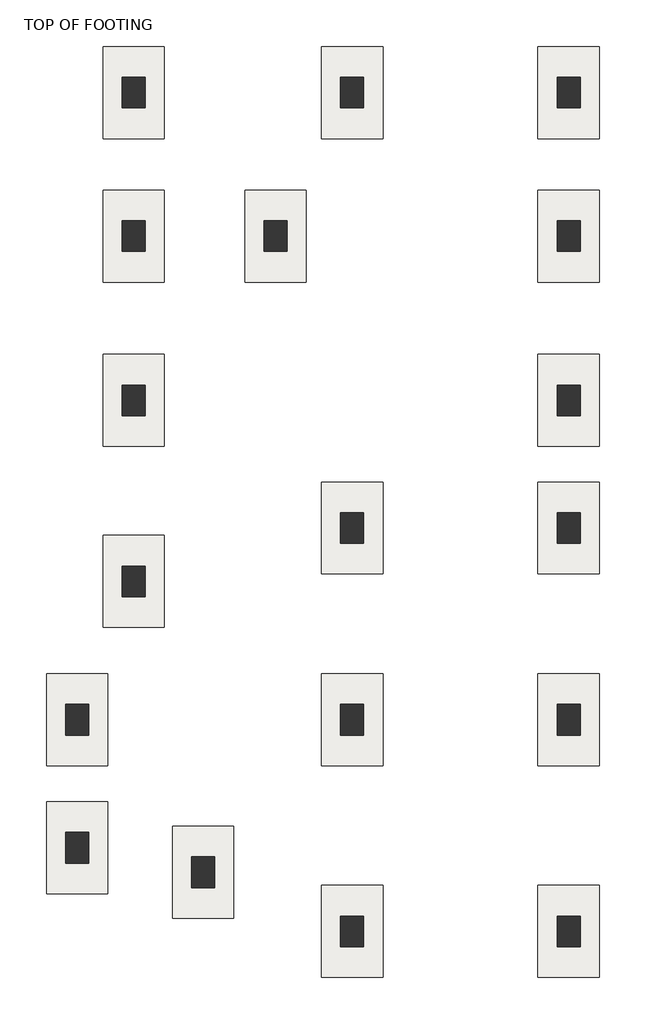
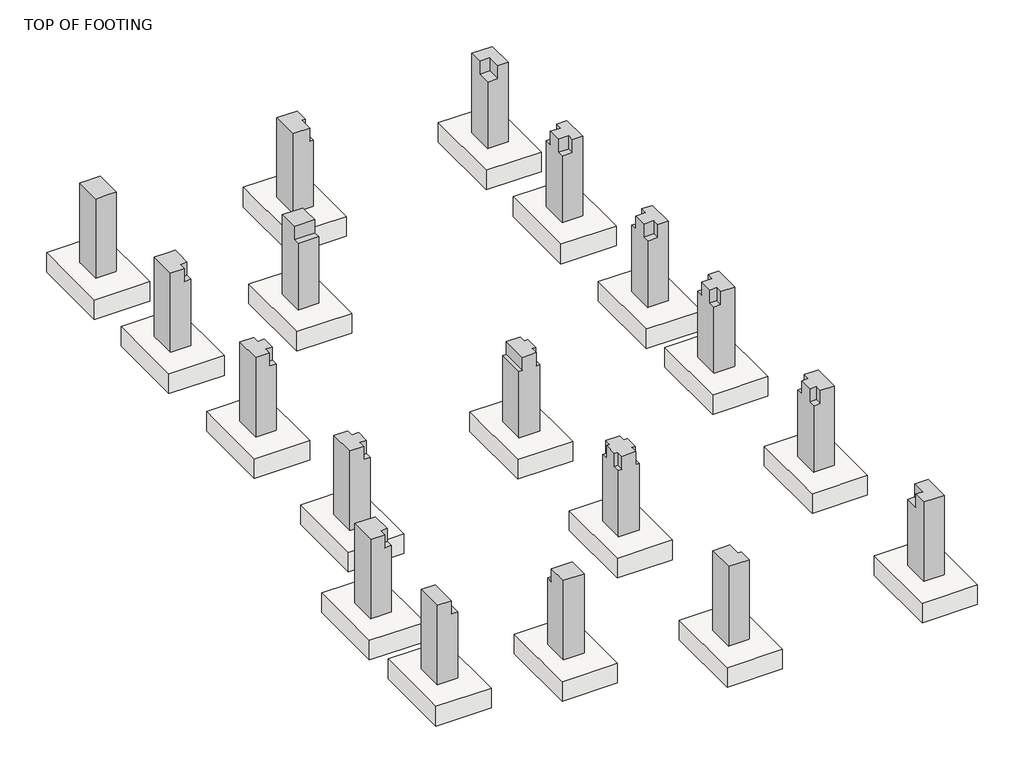
# One storey: 18 columns, 18 slabs.
"""IFC4 building model written with IfcOpenShell, lengths in millimetres."""

from ifc_helpers import new_model, si_unit, frame, origin, place, context, project, spatial, polyline, outline, extrude, faceted_brep, transform, mapped, element, save
from components import m_footing_rectangular_1800_x_1200_x_450mm_16ba7ea5

model = new_model("IFC4")

# Units and contexts
model_context = context("Model", 3, world=origin())
ifc_project = project(units=[si_unit("LENGTHUNIT", "METRE", prefix="MILLI")], contexts=[model_context])

# Site, building, storey
site = spatial("IfcSite", under=ifc_project)
building = spatial("IfcBuilding", under=site)
storey = spatial("IfcBuildingStorey", under=building, Name="TOP OF FOOTING", Elevation=-1828.8)

# Columns
placement = place(None, origin())
element("IfcColumn", 1, ObjectType="M_Concrete-Rectangular-Column : 450 x 600mm", at=placement, inside=storey, context=model_context, shape_type="SweptSolid", body=[
    extrude(outline(polyline([(-1828.8, -7482.9642664), (-1828.8, -7032.9642664), (-300.0, -7032.9642664), (-300.0, -7182.9642664), (0.0, -7182.9642664), (0.0, -7482.9642664), (-1828.8, -7482.9642664)])), frame((0.0, -4929.2575036, 0.0), z_axis=(0.0, 1.0, 0.0), x_axis=(0.0, 0.0, 1.0)), (0.0, 0.0, 1.0), 600.0),
])
element("IfcColumn", 2, ObjectType="M_Concrete-Rectangular-Column : 450 x 600mm", at=placement, inside=storey, context=model_context, shape_type="Brep", body=[
    faceted_brep([(-5925.9642664, 10450.0657956, -1828.8), (-5925.9642664, 9850.0657956, -1828.8), (-6375.9642664, 9850.0657956, -1828.8), (-6375.9642664, 10450.0657956, -1828.8), (-5925.9642664, 10450.0657956, 0.0), (-5925.9642664, 10150.0657956, 0.0), (-5925.9642664, 9850.0657956, 0.0), (-5925.9642664, 9850.0657956, -300.0), (-6075.9642664, 9850.0657956, 0.0), (-6375.9642664, 9850.0657956, 0.0), (-6375.9642664, 10450.0657956, 0.0)], [[[0, 1, 2, 3]], [[1, 0, 4, 5, 6, 7]], [[2, 1, 7, 6, 8, 9]], [[3, 2, 9, 10]], [[0, 3, 10, 4]], [[10, 9, 8, 6, 5, 4]]]),
])
element("IfcColumn", 3, ObjectType="M_Concrete-Rectangular-Column : 450 x 600mm", at=placement, inside=storey, context=model_context, shape_type="Brep", body=[
    faceted_brep([(-5925.9642664, 7641.506653, -1828.8), (-5925.9642664, 7041.506653, -1828.8), (-6375.9642664, 7041.506653, -1828.8), (-6375.9642664, 7641.506653, -1828.8), (-5925.9642664, 7641.506653, -300.0), (-5925.9642664, 7641.506653, 0.0), (-5925.9642664, 7491.506653, 0.0), (-5925.9642664, 7191.506653, 0.0), (-5925.9642664, 7191.506653, -300.0), (-5925.9642664, 7041.506653, -300.0), (-6075.9642664, 7041.506653, -300.0), (-6075.9642664, 7041.506653, 0.0), (-6375.9642664, 7041.506653, 0.0), (-6375.9642664, 7641.506653, 0.0), (-6075.9642664, 7641.506653, 0.0), (-6075.9642664, 7191.506653, 0.0), (-6075.9642664, 7191.506653, -300.0)], [[[0, 1, 2, 3]], [[1, 0, 4, 5, 6, 7, 8, 9]], [[2, 1, 9, 10, 11, 12]], [[3, 2, 12, 13]], [[0, 3, 13, 14, 5, 4]], [[13, 12, 11, 15, 7, 6, 5, 14]], [[16, 10, 9, 8]], [[15, 16, 8, 7]], [[16, 15, 11, 10]]]),
])
element("IfcColumn", 4, ObjectType="M_Concrete-Rectangular-Column : 450 x 600mm", at=placement, inside=storey, context=model_context, shape_type="Brep", body=[
    faceted_brep([(-5925.9642664, 4424.5351605, -1828.8), (-5925.9642664, 3824.5351605, -1828.8), (-6375.9642664, 3824.5351605, -1828.8), (-6375.9642664, 4424.5351605, -1828.8), (-5925.9642664, 4424.5351605, -300.0), (-5925.9642664, 4274.5351605, -300.0), (-5925.9642664, 4274.5351605, 0.0), (-5925.9642664, 3974.5351605, 0.0), (-5925.9642664, 3974.5351605, -300.0), (-5925.9642664, 3824.5351605, -300.0), (-6075.9642664, 3824.5351605, -300.0), (-6075.9642664, 3824.5351605, 0.0), (-6375.9642664, 3824.5351605, 0.0), (-6375.9642664, 4424.5351605, 0.0), (-6075.9642664, 4424.5351605, 0.0), (-6075.9642664, 4424.5351605, -300.0), (-6075.9642664, 3974.5351605, 0.0), (-6075.9642664, 4274.5351605, 0.0), (-6075.9642664, 4274.5351605, -300.0), (-6075.9642664, 3974.5351605, -300.0)], [[[0, 1, 2, 3]], [[1, 0, 4, 5, 6, 7, 8, 9]], [[2, 1, 9, 10, 11, 12]], [[3, 2, 12, 13]], [[0, 3, 13, 14, 15, 4]], [[13, 12, 11, 16, 7, 6, 17, 14]], [[15, 18, 5, 4]], [[18, 17, 6, 5]], [[17, 18, 15, 14]], [[19, 10, 9, 8]], [[16, 19, 8, 7]], [[19, 16, 11, 10]]]),
])
element("IfcColumn", 5, ObjectType="M_Concrete-Rectangular-Column : 450 x 600mm", at=placement, inside=storey, context=model_context, shape_type="Brep", body=[
    faceted_brep([(-5925.9642664, 881.5941646, -1828.8), (-5925.9642664, 281.5941646, -1828.8), (-6375.9642664, 281.5941646, -1828.8), (-6375.9642664, 881.5941646, -1828.8), (-5925.9642664, 881.5941646, -300.0), (-5925.9642664, 731.5941646, -300.0), (-5925.9642664, 731.5941646, 0.0), (-5925.9642664, 431.5941646, 0.0), (-5925.9642664, 431.5941646, -300.0), (-5925.9642664, 281.5941646, -300.0), (-6075.9642664, 281.5941646, -300.0), (-6075.9642664, 281.5941646, 0.0), (-6375.9642664, 281.5941646, 0.0), (-6375.9642664, 881.5941646, 0.0), (-6075.9642664, 881.5941646, 0.0), (-6075.9642664, 881.5941646, -300.0), (-6075.9642664, 431.5941646, 0.0), (-6075.9642664, 731.5941646, 0.0), (-6075.9642664, 731.5941646, -300.0), (-6075.9642664, 431.5941646, -300.0)], [[[0, 1, 2, 3]], [[1, 0, 4, 5, 6, 7, 8, 9]], [[2, 1, 9, 10, 11, 12]], [[3, 2, 12, 13]], [[0, 3, 13, 14, 15, 4]], [[13, 12, 11, 16, 7, 6, 17, 14]], [[15, 18, 5, 4]], [[18, 17, 6, 5]], [[17, 18, 15, 14]], [[19, 10, 9, 8]], [[19, 16, 11, 10]], [[16, 19, 8, 7]]]),
])
element("IfcColumn", 6, ObjectType="M_Concrete-Rectangular-Column : 450 x 600mm", at=placement, inside=storey, context=model_context, shape_type="Brep", body=[
    faceted_brep([(-3146.635935, 7641.506653, -1828.8), (-3146.635935, 7041.506653, -1828.8), (-3596.635935, 7041.506653, -1828.8), (-3596.635935, 7641.506653, -1828.8), (-3146.635935, 7641.506653, -300.0), (-3146.635935, 7641.506653, 0.0), (-3146.635935, 7491.506653, 0.0), (-3146.635935, 7191.506653, 0.0), (-3146.635935, 7191.506653, -300.0), (-3146.635935, 7041.506653, -300.0), (-3596.635935, 7041.506653, -300.0), (-3596.635935, 7191.506653, -300.0), (-3596.635935, 7191.506653, 0.0), (-3596.635935, 7491.506653, 0.0), (-3596.635935, 7641.506653, 0.0), (-3596.635935, 7641.506653, -300.0)], [[[0, 1, 2, 3]], [[1, 0, 4, 5, 6, 7, 8, 9]], [[2, 1, 9, 10]], [[3, 2, 10, 11, 12, 13, 14, 15]], [[0, 3, 15, 14, 5, 4]], [[5, 14, 13, 12, 7, 6]], [[8, 11, 10, 9]], [[11, 8, 7, 12]]]),
])
element("IfcColumn", 7, ObjectType="M_Concrete-Rectangular-Column : 450 x 600mm", at=placement, inside=storey, context=model_context, shape_type="Brep", body=[
    faceted_brep([(-1646.635935, 10450.0657956, -1828.8), (-1646.635935, 9850.0657956, -1828.8), (-2096.635935, 9850.0657956, -1828.8), (-2096.635935, 10450.0657956, -1828.8), (-1646.635935, 10450.0657956, 0.0), (-1646.635935, 10150.0657956, 0.0), (-1646.635935, 10150.0657956, -300.0), (-1646.635935, 9850.0657956, -300.0), (-1721.635935, 9850.0657956, -300.0), (-1721.635935, 9850.0657956, 0.0), (-2021.635935, 9850.0657956, 0.0), (-2096.635935, 9850.0657956, 0.0), (-2096.635935, 9850.0657956, -300.0), (-2096.635935, 10150.0657956, 0.0), (-2096.635935, 10450.0657956, 0.0), (-1721.635935, 10150.0657956, 0.0), (-1721.635935, 10150.0657956, -300.0)], [[[0, 1, 2, 3]], [[1, 0, 4, 5, 6, 7]], [[2, 1, 7, 8, 9, 10, 11, 12]], [[3, 2, 12, 11, 13, 14]], [[0, 3, 14, 4]], [[4, 14, 13, 11, 10, 9, 15, 5]], [[16, 8, 7, 6]], [[15, 16, 6, 5]], [[16, 15, 9, 8]]]),
])
element("IfcColumn", 8, ObjectType="M_Concrete-Rectangular-Column : 450 x 600mm", at=placement, inside=storey, context=model_context, shape_type="Brep", body=[
    faceted_brep([(-1646.635935, 1928.1057379, -1828.8), (-1646.635935, 1328.1057379, -1828.8), (-2096.635935, 1328.1057379, -1828.8), (-2096.635935, 1928.1057379, -1828.8), (-1646.635935, 1928.1057379, -300.0), (-1646.635935, 1778.1057379, -300.0), (-1646.635935, 1778.1057379, 0.0), (-1646.635935, 1478.1057379, 0.0), (-1646.635935, 1478.1057379, -300.0), (-1646.635935, 1328.1057379, -300.0), (-1721.635935, 1328.1057379, -300.0), (-1721.635935, 1328.1057379, 0.0), (-2021.635935, 1328.1057379, 0.0), (-2021.635935, 1328.1057379, -300.0), (-2096.635935, 1328.1057379, -300.0), (-2096.635935, 1928.1057379, -300.0), (-2021.635935, 1928.1057379, -300.0), (-2021.635935, 1928.1057379, 0.0), (-1721.635935, 1928.1057379, 0.0), (-1721.635935, 1928.1057379, -300.0), (-1721.635935, 1778.1057379, 0.0), (-1721.635935, 1478.1057379, 0.0), (-1721.635935, 1778.1057379, -300.0), (-1721.635935, 1478.1057379, -300.0)], [[[0, 1, 2, 3]], [[1, 0, 4, 5, 6, 7, 8, 9]], [[2, 1, 9, 10, 11, 12, 13, 14]], [[3, 2, 14, 15]], [[0, 3, 15, 16, 17, 18, 19, 4]], [[6, 20, 18, 17, 12, 11, 21, 7]], [[19, 22, 5, 4]], [[22, 20, 6, 5]], [[20, 22, 19, 18]], [[23, 10, 9, 8]], [[21, 23, 8, 7]], [[23, 21, 11, 10]], [[13, 16, 15, 14]], [[16, 13, 12, 17]]]),
])
element("IfcColumn", 9, ObjectType="M_Concrete-Rectangular-Column : 450 x 600mm", at=placement, inside=storey, context=model_context, shape_type="Brep", body=[
    faceted_brep([(-1646.635935, -1823.3693625, -1828.8), (-1646.635935, -2423.3693625, -1828.8), (-2096.635935, -2423.3693625, -1828.8), (-2096.635935, -1823.3693625, -1828.8), (-1646.635935, -1823.3693625, -300.0), (-1646.635935, -1973.3693625, -300.0), (-1646.635935, -1973.3693625, 0.0), (-1646.635935, -2273.3693625, 0.0), (-1646.635935, -2273.3693625, -300.0), (-1646.635935, -2423.3693625, -300.0), (-1721.635935, -2423.3693625, -300.0), (-1721.635935, -2423.3693625, 0.0), (-2021.635935, -2423.3693625, 0.0), (-2021.635935, -2423.3693625, -300.0), (-2096.635935, -2423.3693625, -300.0), (-2096.635935, -2273.3693625, -300.0), (-2096.635935, -2273.3693625, 0.0), (-2096.635935, -1973.3693625, 0.0), (-2096.635935, -1973.3693625, -300.0), (-2096.635935, -1823.3693625, -300.0), (-2021.635935, -1823.3693625, -300.0), (-2021.635935, -1823.3693625, 0.0), (-1721.635935, -1823.3693625, 0.0), (-1721.635935, -1823.3693625, -300.0), (-1721.635935, -1973.3693625, 0.0), (-2021.635935, -1973.3693625, 0.0), (-2021.635935, -2273.3693625, 0.0), (-1721.635935, -2273.3693625, 0.0), (-1721.635935, -1973.3693625, -300.0), (-1721.635935, -2273.3693625, -300.0), (-2021.635935, -1973.3693625, -300.0), (-2021.635935, -2273.3693625, -300.0)], [[[0, 1, 2, 3]], [[1, 0, 4, 5, 6, 7, 8, 9]], [[2, 1, 9, 10, 11, 12, 13, 14]], [[3, 2, 14, 15, 16, 17, 18, 19]], [[0, 3, 19, 20, 21, 22, 23, 4]], [[6, 24, 22, 21, 25, 17, 16, 26, 12, 11, 27, 7]], [[23, 28, 5, 4]], [[28, 24, 6, 5]], [[24, 28, 23, 22]], [[29, 10, 9, 8]], [[27, 29, 8, 7]], [[29, 27, 11, 10]], [[18, 30, 20, 19]], [[30, 25, 21, 20]], [[25, 30, 18, 17]], [[13, 31, 15, 14]], [[31, 26, 16, 15]], [[26, 31, 13, 12]]]),
])
element("IfcColumn", 10, ObjectType="M_Concrete-Rectangular-Column : 450 x 600mm", at=placement, inside=storey, context=model_context, shape_type="Brep", body=[
    faceted_brep([(-1646.635935, -5967.3380763, -1828.8), (-1646.635935, -6567.3380763, -1828.8), (-2096.635935, -6567.3380763, -1828.8), (-2096.635935, -5967.3380763, -1828.8), (-1646.635935, -5967.3380763, -300.0), (-1646.635935, -6267.3380763, -300.0), (-1646.635935, -6267.3380763, 0.0), (-1646.635935, -6567.3380763, 0.0), (-2096.635935, -6567.3380763, 0.0), (-2096.635935, -5967.3380763, 0.0), (-1721.635935, -5967.3380763, 0.0), (-1721.635935, -5967.3380763, -300.0), (-1721.635935, -6267.3380763, 0.0), (-1721.635935, -6267.3380763, -300.0)], [[[0, 1, 2, 3]], [[1, 0, 4, 5, 6, 7]], [[2, 1, 7, 8]], [[3, 2, 8, 9]], [[0, 3, 9, 10, 11, 4]], [[8, 7, 6, 12, 10, 9]], [[11, 13, 5, 4]], [[13, 12, 6, 5]], [[12, 13, 11, 10]]]),
])
element("IfcColumn", 11, ObjectType="M_Concrete-Rectangular-Column : 450 x 600mm", at=placement, inside=storey, context=model_context, shape_type="Brep", body=[
    faceted_brep([(2593.5134108, 10450.0657956, -1828.8), (2593.5134108, 9850.0657956, -1828.8), (2143.5134108, 9850.0657956, -1828.8), (2143.5134108, 10450.0657956, -1828.8), (2593.5134108, 10450.0657956, 0.0), (2593.5134108, 9850.0657956, 0.0), (2368.5134108, 9850.0657956, 0.0), (2368.5134108, 9850.0657956, -300.0), (2143.5134108, 9850.0657956, -300.0), (2143.5134108, 10150.0657956, -300.0), (2143.5134108, 10150.0657956, 0.0), (2143.5134108, 10450.0657956, 0.0), (2368.5134108, 10150.0657956, 0.0), (2368.5134108, 10150.0657956, -300.0)], [[[0, 1, 2, 3]], [[1, 0, 4, 5]], [[2, 1, 5, 6, 7, 8]], [[3, 2, 8, 9, 10, 11]], [[0, 3, 11, 4]], [[5, 4, 11, 10, 12, 6]], [[7, 13, 9, 8]], [[13, 12, 10, 9]], [[12, 13, 7, 6]]]),
])
element("IfcColumn", 12, ObjectType="M_Concrete-Rectangular-Column : 450 x 600mm", at=placement, inside=storey, context=model_context, shape_type="Brep", body=[
    faceted_brep([(2593.5134108, 7641.506653, -1828.8), (2593.5134108, 7041.506653, -1828.8), (2143.5134108, 7041.506653, -1828.8), (2143.5134108, 7641.506653, -1828.8), (2593.5134108, 7641.506653, 0.0), (2593.5134108, 7041.506653, 0.0), (2368.5134108, 7041.506653, 0.0), (2368.5134108, 7041.506653, -300.0), (2143.5134108, 7041.506653, -300.0), (2143.5134108, 7191.506653, -300.0), (2143.5134108, 7191.506653, 0.0), (2143.5134108, 7491.506653, 0.0), (2143.5134108, 7491.506653, -300.0), (2143.5134108, 7641.506653, -300.0), (2368.5134108, 7641.506653, -300.0), (2368.5134108, 7641.506653, 0.0), (2368.5134108, 7491.506653, 0.0), (2368.5134108, 7191.506653, 0.0), (2368.5134108, 7491.506653, -300.0), (2368.5134108, 7191.506653, -300.0)], [[[0, 1, 2, 3]], [[1, 0, 4, 5]], [[2, 1, 5, 6, 7, 8]], [[3, 2, 8, 9, 10, 11, 12, 13]], [[0, 3, 13, 14, 15, 4]], [[5, 4, 15, 16, 11, 10, 17, 6]], [[12, 18, 14, 13]], [[18, 16, 15, 14]], [[16, 18, 12, 11]], [[7, 19, 9, 8]], [[19, 17, 10, 9]], [[17, 19, 7, 6]]]),
])
element("IfcColumn", 13, ObjectType="M_Concrete-Rectangular-Column : 450 x 600mm", at=placement, inside=storey, context=model_context, shape_type="Brep", body=[
    faceted_brep([(2593.5134108, 4424.5351605, -1828.8), (2593.5134108, 3824.5351605, -1828.8), (2143.5134108, 3824.5351605, -1828.8), (2143.5134108, 4424.5351605, -1828.8), (2593.5134108, 4424.5351605, 0.0), (2593.5134108, 3824.5351605, 0.0), (2368.5134108, 3824.5351605, 0.0), (2368.5134108, 3824.5351605, -300.0), (2143.5134108, 3824.5351605, -300.0), (2143.5134108, 3974.5351605, -300.0), (2143.5134108, 3974.5351605, 0.0), (2143.5134108, 4274.5351605, 0.0), (2143.5134108, 4274.5351605, -300.0), (2143.5134108, 4424.5351605, -300.0), (2368.5134108, 4424.5351605, -300.0), (2368.5134108, 4424.5351605, 0.0), (2368.5134108, 4274.5351605, 0.0), (2368.5134108, 3974.5351605, 0.0), (2368.5134108, 4274.5351605, -300.0), (2368.5134108, 3974.5351605, -300.0)], [[[0, 1, 2, 3]], [[1, 0, 4, 5]], [[2, 1, 5, 6, 7, 8]], [[3, 2, 8, 9, 10, 11, 12, 13]], [[0, 3, 13, 14, 15, 4]], [[5, 4, 15, 16, 11, 10, 17, 6]], [[12, 18, 14, 13]], [[18, 16, 15, 14]], [[16, 18, 12, 11]], [[7, 19, 9, 8]], [[17, 19, 7, 6]], [[19, 17, 10, 9]]]),
])
element("IfcColumn", 14, ObjectType="M_Concrete-Rectangular-Column : 450 x 600mm", at=placement, inside=storey, context=model_context, shape_type="Brep", body=[
    faceted_brep([(2593.5134108, 1928.1057379, -1828.8), (2593.5134108, 1328.1057379, -1828.8), (2143.5134108, 1328.1057379, -1828.8), (2143.5134108, 1928.1057379, -1828.8), (2593.5134108, 1928.1057379, 0.0), (2593.5134108, 1328.1057379, 0.0), (2293.5134108, 1328.1057379, 0.0), (2293.5134108, 1328.1057379, -300.0), (2143.5134108, 1328.1057379, -300.0), (2143.5134108, 1478.1057379, -300.0), (2143.5134108, 1478.1057379, 0.0), (2143.5134108, 1778.1057379, 0.0), (2143.5134108, 1778.1057379, -300.0), (2143.5134108, 1928.1057379, -300.0), (2368.5134108, 1928.1057379, -300.0), (2368.5134108, 1928.1057379, 0.0), (2368.5134108, 1778.1057379, 0.0), (2293.5134108, 1478.1057379, 0.0), (2368.5134108, 1778.1057379, -300.0), (2293.5134108, 1478.1057379, -300.0)], [[[0, 1, 2, 3]], [[1, 0, 4, 5]], [[2, 1, 5, 6, 7, 8]], [[3, 2, 8, 9, 10, 11, 12, 13]], [[0, 3, 13, 14, 15, 4]], [[5, 4, 15, 16, 11, 10, 17, 6]], [[12, 18, 14, 13]], [[18, 16, 15, 14]], [[16, 18, 12, 11]], [[7, 19, 9, 8]], [[19, 17, 10, 9]], [[17, 19, 7, 6]]]),
])
element("IfcColumn", 15, ObjectType="M_Concrete-Rectangular-Column : 450 x 600mm", at=placement, inside=storey, context=model_context, shape_type="Brep", body=[
    faceted_brep([(2593.5134108, -1823.3693625, -1828.8), (2593.5134108, -2423.3693625, -1828.8), (2143.5134108, -2423.3693625, -1828.8), (2143.5134108, -1823.3693625, -1828.8), (2593.5134108, -1823.3693625, 0.0), (2593.5134108, -2423.3693625, 0.0), (2293.5134108, -2423.3693625, 0.0), (2293.5134108, -2423.3693625, -300.0), (2143.5134108, -2423.3693625, -300.0), (2143.5134108, -2273.3693625, -300.0), (2143.5134108, -2273.3693625, 0.0), (2143.5134108, -1973.3693625, 0.0), (2143.5134108, -1973.3693625, -300.0), (2143.5134108, -1823.3693625, -300.0), (2293.5134108, -1823.3693625, -300.0), (2293.5134108, -1823.3693625, 0.0), (2293.5134108, -1973.3693625, 0.0), (2293.5134108, -2273.3693625, 0.0), (2293.5134108, -1973.3693625, -300.0), (2293.5134108, -2273.3693625, -300.0)], [[[0, 1, 2, 3]], [[1, 0, 4, 5]], [[2, 1, 5, 6, 7, 8]], [[3, 2, 8, 9, 10, 11, 12, 13]], [[0, 3, 13, 14, 15, 4]], [[5, 4, 15, 16, 11, 10, 17, 6]], [[12, 18, 14, 13]], [[18, 16, 15, 14]], [[16, 18, 12, 11]], [[7, 19, 9, 8]], [[19, 17, 10, 9]], [[17, 19, 7, 6]]]),
])
element("IfcColumn", 16, ObjectType="M_Concrete-Rectangular-Column : 450 x 600mm", at=placement, inside=storey, context=model_context, shape_type="Brep", body=[
    faceted_brep([(2593.5134108, -5967.3380763, -1828.8), (2593.5134108, -6567.3380763, -1828.8), (2143.5134108, -6567.3380763, -1828.8), (2143.5134108, -5967.3380763, -1828.8), (2593.5134108, -5967.3380763, 0.0), (2593.5134108, -6567.3380763, 0.0), (2143.5134108, -6567.3380763, 0.0), (2143.5134108, -6267.3380763, 0.0), (2143.5134108, -6267.3380763, -300.0), (2143.5134108, -5967.3380763, -300.0), (2293.5134108, -5967.3380763, -300.0), (2293.5134108, -5967.3380763, 0.0), (2293.5134108, -6267.3380763, 0.0), (2293.5134108, -6267.3380763, -300.0)], [[[0, 1, 2, 3]], [[1, 0, 4, 5]], [[2, 1, 5, 6]], [[3, 2, 6, 7, 8, 9]], [[0, 3, 9, 10, 11, 4]], [[5, 4, 11, 12, 7, 6]], [[8, 13, 10, 9]], [[13, 12, 11, 10]], [[12, 13, 8, 7]]]),
])
element("IfcColumn", 17, ObjectType="M_Concrete-Rectangular-Column : 450 x 600mm", at=placement, inside=storey, context=model_context, shape_type="SweptSolid", body=[
    extrude(outline(polyline([(-4809.2575036, -1828.8), (-5409.2575036, -1828.8), (-5409.2575036, 0.0), (-4959.2575036, 0.0), (-4959.2575036, -300.0), (-4809.2575036, -300.0), (-4809.2575036, -1828.8)])), frame((-5016.635935, 0.0, 0.0), z_axis=(1.0, 0.0, 0.0), x_axis=(0.0, 1.0, 0.0)), (0.0, 0.0, 1.0), 450.0),
])
element("IfcColumn", 18, ObjectType="M_Concrete-Rectangular-Column : 450 x 600mm", at=placement, inside=storey, context=model_context, shape_type="Brep", body=[
    faceted_brep([(-7032.9642664, -1823.3693625, -1828.8), (-7032.9642664, -2423.3693625, -1828.8), (-7482.9642664, -2423.3693625, -1828.8), (-7482.9642664, -1823.3693625, -1828.8), (-7032.9642664, -1823.3693625, 0.0), (-7032.9642664, -2273.3693625, 0.0), (-7032.9642664, -2273.3693625, -300.0), (-7032.9642664, -2423.3693625, -300.0), (-7182.9642664, -2423.3693625, -300.0), (-7182.9642664, -2423.3693625, 0.0), (-7482.9642664, -2423.3693625, 0.0), (-7482.9642664, -1823.3693625, 0.0), (-7182.9642664, -2273.3693625, 0.0), (-7182.9642664, -2273.3693625, -300.0)], [[[0, 1, 2, 3]], [[1, 0, 4, 5, 6, 7]], [[2, 1, 7, 8, 9, 10]], [[3, 2, 10, 11]], [[0, 3, 11, 4]], [[11, 10, 9, 12, 5, 4]], [[13, 8, 7, 6]], [[12, 13, 6, 5]], [[13, 12, 9, 8]]]),
])

# Slabs
m_footing_rectangular_1800_x_1200_x_450mm_shape = m_footing_rectangular_1800_x_1200_x_450mm_16ba7ea5(model_context)
element("IfcSlab", 19, ObjectType="M_Footing-Rectangular : 1800 x 1200 x 450mm", at=placement, inside=storey, context=model_context, shape_type="MappedRepresentation", body=[
    mapped(m_footing_rectangular_1800_x_1200_x_450mm_shape, transform((-7257.9642664, -4629.2575036, -1828.8), x_axis=(1.0, 0.0, 0.0), y_axis=(0.0, 1.0, 0.0), z_axis=(0.0, 0.0, 1.0))),
])
element("IfcSlab", 20, ObjectType="M_Footing-Rectangular : 1800 x 1200 x 450mm", at=placement, inside=storey, context=model_context, shape_type="MappedRepresentation", body=[
    mapped(m_footing_rectangular_1800_x_1200_x_450mm_shape, transform((-4791.635935, -5109.2575036, -1828.8), x_axis=(1.0, 0.0, 0.0), y_axis=(0.0, 1.0, 0.0), z_axis=(0.0, 0.0, 1.0))),
])
element("IfcSlab", 21, ObjectType="M_Footing-Rectangular : 1800 x 1200 x 450mm", at=placement, inside=storey, context=model_context, shape_type="MappedRepresentation", body=[
    mapped(m_footing_rectangular_1800_x_1200_x_450mm_shape, transform((2368.5134108, -6267.3380763, -1828.8), x_axis=(1.0, 0.0, 0.0), y_axis=(0.0, 1.0, 0.0), z_axis=(0.0, 0.0, 1.0))),
])
element("IfcSlab", 22, ObjectType="M_Footing-Rectangular : 1800 x 1200 x 450mm", at=placement, inside=storey, context=model_context, shape_type="MappedRepresentation", body=[
    mapped(m_footing_rectangular_1800_x_1200_x_450mm_shape, transform((-1871.635935, -6267.3380763, -1828.8), x_axis=(1.0, 0.0, 0.0), y_axis=(0.0, 1.0, 0.0), z_axis=(0.0, 0.0, 1.0))),
])
element("IfcSlab", 23, ObjectType="M_Footing-Rectangular : 1800 x 1200 x 450mm", at=placement, inside=storey, context=model_context, shape_type="MappedRepresentation", body=[
    mapped(m_footing_rectangular_1800_x_1200_x_450mm_shape, transform((2368.5134108, -2123.3693625, -1828.8), x_axis=(1.0, 0.0, 0.0), y_axis=(0.0, 1.0, 0.0), z_axis=(0.0, 0.0, 1.0))),
])
element("IfcSlab", 24, ObjectType="M_Footing-Rectangular : 1800 x 1200 x 450mm", at=placement, inside=storey, context=model_context, shape_type="MappedRepresentation", body=[
    mapped(m_footing_rectangular_1800_x_1200_x_450mm_shape, transform((2368.5134108, 4124.5351605, -1828.8), x_axis=(1.0, 0.0, 0.0), y_axis=(0.0, 1.0, 0.0), z_axis=(0.0, 0.0, 1.0))),
])
element("IfcSlab", 25, ObjectType="M_Footing-Rectangular : 1800 x 1200 x 450mm", at=placement, inside=storey, context=model_context, shape_type="MappedRepresentation", body=[
    mapped(m_footing_rectangular_1800_x_1200_x_450mm_shape, transform((2368.5134108, 10150.0657956, -1828.8), x_axis=(1.0, 0.0, 0.0), y_axis=(0.0, 1.0, 0.0), z_axis=(0.0, 0.0, 1.0))),
])
element("IfcSlab", 26, ObjectType="M_Footing-Rectangular : 1800 x 1200 x 450mm", at=placement, inside=storey, context=model_context, shape_type="MappedRepresentation", body=[
    mapped(m_footing_rectangular_1800_x_1200_x_450mm_shape, transform((-6150.9642664, 10150.0657956, -1828.8), x_axis=(1.0, 0.0, 0.0), y_axis=(0.0, 1.0, 0.0), z_axis=(0.0, 0.0, 1.0))),
])
element("IfcSlab", 27, ObjectType="M_Footing-Rectangular : 1800 x 1200 x 450mm", at=placement, inside=storey, context=model_context, shape_type="MappedRepresentation", body=[
    mapped(m_footing_rectangular_1800_x_1200_x_450mm_shape, transform((-1871.635935, 10150.0657956, -1828.8), x_axis=(1.0, 0.0, 0.0), y_axis=(0.0, 1.0, 0.0), z_axis=(0.0, 0.0, 1.0))),
])
element("IfcSlab", 28, ObjectType="M_Footing-Rectangular : 1800 x 1200 x 450mm", at=placement, inside=storey, context=model_context, shape_type="MappedRepresentation", body=[
    mapped(m_footing_rectangular_1800_x_1200_x_450mm_shape, transform((-6150.9642664, 581.5941646, -1828.8), x_axis=(1.0, 0.0, 0.0), y_axis=(0.0, 1.0, 0.0), z_axis=(0.0, 0.0, 1.0))),
])
element("IfcSlab", 29, ObjectType="M_Footing-Rectangular : 1800 x 1200 x 450mm", at=placement, inside=storey, context=model_context, shape_type="MappedRepresentation", body=[
    mapped(m_footing_rectangular_1800_x_1200_x_450mm_shape, transform((-6150.9642664, 4124.5351605, -1828.8), x_axis=(1.0, 0.0, 0.0), y_axis=(0.0, 1.0, 0.0), z_axis=(0.0, 0.0, 1.0))),
])
element("IfcSlab", 30, ObjectType="M_Footing-Rectangular : 1800 x 1200 x 450mm", at=placement, inside=storey, context=model_context, shape_type="MappedRepresentation", body=[
    mapped(m_footing_rectangular_1800_x_1200_x_450mm_shape, transform((-6150.9642664, 7341.506653, -1828.8), x_axis=(1.0, 0.0, 0.0), y_axis=(0.0, 1.0, 0.0), z_axis=(0.0, 0.0, 1.0))),
])
element("IfcSlab", 31, ObjectType="M_Footing-Rectangular : 1800 x 1200 x 450mm", at=placement, inside=storey, context=model_context, shape_type="MappedRepresentation", body=[
    mapped(m_footing_rectangular_1800_x_1200_x_450mm_shape, transform((-3371.635935, 7341.506653, -1828.8), x_axis=(1.0, 0.0, 0.0), y_axis=(0.0, 1.0, 0.0), z_axis=(0.0, 0.0, 1.0))),
])
element("IfcSlab", 32, ObjectType="M_Footing-Rectangular : 1800 x 1200 x 450mm", at=placement, inside=storey, context=model_context, shape_type="MappedRepresentation", body=[
    mapped(m_footing_rectangular_1800_x_1200_x_450mm_shape, transform((2368.5134108, 7341.506653, -1828.8), x_axis=(1.0, 0.0, 0.0), y_axis=(0.0, 1.0, 0.0), z_axis=(0.0, 0.0, 1.0))),
])
element("IfcSlab", 33, ObjectType="M_Footing-Rectangular : 1800 x 1200 x 450mm", at=placement, inside=storey, context=model_context, shape_type="MappedRepresentation", body=[
    mapped(m_footing_rectangular_1800_x_1200_x_450mm_shape, transform((-1871.635935, -2123.3693625, -1828.8), x_axis=(1.0, 0.0, 0.0), y_axis=(0.0, 1.0, 0.0), z_axis=(0.0, 0.0, 1.0))),
])
element("IfcSlab", 34, ObjectType="M_Footing-Rectangular : 1800 x 1200 x 450mm", at=placement, inside=storey, context=model_context, shape_type="MappedRepresentation", body=[
    mapped(m_footing_rectangular_1800_x_1200_x_450mm_shape, transform((2368.5134108, 1628.1057379, -1828.8), x_axis=(1.0, 0.0, 0.0), y_axis=(0.0, 1.0, 0.0), z_axis=(0.0, 0.0, 1.0))),
])
element("IfcSlab", 35, ObjectType="M_Footing-Rectangular : 1800 x 1200 x 450mm", at=placement, inside=storey, context=model_context, shape_type="MappedRepresentation", body=[
    mapped(m_footing_rectangular_1800_x_1200_x_450mm_shape, transform((-1871.635935, 1628.1057379, -1828.8), x_axis=(1.0, 0.0, 0.0), y_axis=(0.0, 1.0, 0.0), z_axis=(0.0, 0.0, 1.0))),
])
element("IfcSlab", 36, ObjectType="M_Footing-Rectangular : 1800 x 1200 x 450mm", at=placement, inside=storey, context=model_context, shape_type="MappedRepresentation", body=[
    mapped(m_footing_rectangular_1800_x_1200_x_450mm_shape, transform((-7257.9642664, -2123.3693625, -1828.8), x_axis=(1.0, 0.0, 0.0), y_axis=(0.0, 1.0, 0.0), z_axis=(0.0, 0.0, 1.0))),
])

save(model, "model.ifc")

# Revit data of these elements
# Grids (mm)
#   "9": line (6345.331, -5109.258) -> (-9404.782, -5109.258)
#   "10": line (6345.331, -6267.338) -> (-9427.998, -6267.338)
#   "1": line (6418.05, 10150.066) -> (-9427.998, 10150.066)
#   "A": line (-7257.964, 12244.334) -> (-7257.964, -11102.212)
#   "B": line (-6150.964, 12244.334) -> (-6150.964, -11102.212)
#   "C": line (-4791.636, 12244.334) -> (-4791.636, -8322.372)
#   "D": line (-3371.636, 12244.334) -> (-3371.636, -8322.372)
#   "2": line (6418.05, 7341.507) -> (-9427.998, 7341.507)
#   "E": line (-1871.636, 12244.334) -> (-1871.636, -8322.372)
#   "F": line (2368.513, 12244.334) -> (2368.513, -8382.306)
#   "8": line (6418.05, -4629.258) -> (-9404.782, -4629.258)
#   "3": line (6418.05, 6151.507) -> (-9427.998, 6151.507)
#   "G": line (3608.513, 12244.334) -> (3608.513, -8322.372)
#   "4": line (6418.05, 4124.535) -> (-9404.782, 4124.535)
#   "5": line (6345.331, 1628.106) -> (-9404.782, 1628.106)
#   "6": line (6345.331, 581.594) -> (-9427.998, 581.594)
#   "7": line (6418.05, -2123.369) -> (-9404.782, -2123.369)
# Type "M_Concrete-Rectangular-Column : 450 x 600mm"
#   b = 450 mm
#   h = 600 mm
#   Structural Material [instance default] = Concrete, Cast-in-Place gray
# Type "M_Footing-Rectangular : 1800 x 1200 x 450mm"
#   Width = 1200 mm
#   Length = 1800 mm
#   Foundation Thickness = 450 mm
#   Structural Material [instance default] = Concrete, Cast-in-Place gray
#   Assembly Code = ""
# Elements 1, 2, 3, 4, 5, 6, 7, 8, 9, 10, 11, 12, 13, 14, 15, 16, 17, 18 (IfcColumn, "M_Concrete-Rectangular-Column : 450 x 600mm")
#   Structural Material = Concrete, Cast-in-Place gray
#   Phase Created = New Construction
#   Materials on its faces: "Concrete, Cast-in-Place gray"
# Elements 19, 20, 21, 22, 23, 24, 25, 26, 27, 28, 29, 30, 31, 32, 33, 34, 35, 36 (IfcSlab, "M_Footing-Rectangular : 1800 x 1200 x 450mm")
#   Structural Material = Concrete, Cast-in-Place gray
#   Phase Created = New Construction
#   Materials on its faces: "Concrete, Cast-in-Place gray"
# Materials
#   "Concrete, Cast-in-Place gray": class "Concrete", colour RGB 192 192 192, transparency 0, Description = "Cast-in-place concrete", Cost = 0
